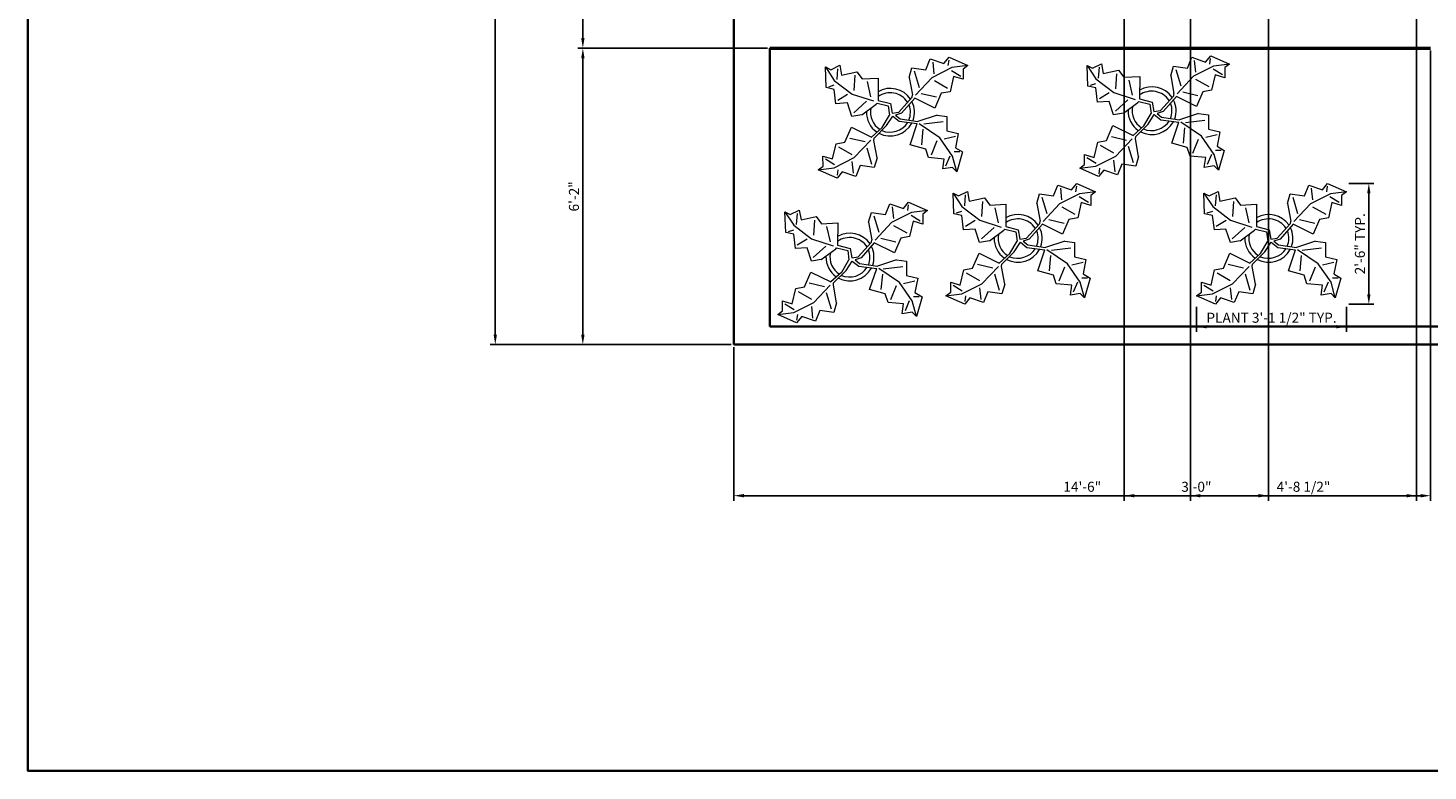
# Model space of a CAD drawing. Units: inches. Extents: x 65 to 818, y -87 to 880.
# Tile 1 of 6: x 65 to 414, y -87 to 98. Entities that reach past the tile are written whole.
import ezdxf

# ---------------------------------------------------------------- set-up
doc = ezdxf.new("R2010")
doc.units = ezdxf.units.IN
for name, color, linetype, lineweight in [('A-ANNO-DIMS', 2, 'Continuous', 18), ('A-ANNO-TTLB', 7, 'Continuous', 35), ('A-WALL', 7, 'Continuous', 50), ('C-PROP', 7, 'Continuous', 35), ('L-PLNT', 94, 'Continuous', 13)]:
    doc.layers.add(name, color=color, linetype=linetype, lineweight=lineweight)
doc.styles.get("Standard").update_dxf_attribs({"font": 'arial.ttf'})
doc.dimstyles.new('ISO-25', dxfattribs={"dimtxt": 2.5, "dimasz": 2.5, "dimexe": 1.25, "dimexo": 0.625, "dimtad": 1, "dimtxsty": 'Standard', "dimcen": 2.5, "dimadec": 0, "dimazin": 0, "dimtfac": 1, "dimtmove": 0, "dimatfit": 3, "dimfxl": 1, "dimarcsym": 0})

# ---------------------------------------------------------------- blocks, each defined once
blk = doc.blocks.new('Plant - Rubber or Philodendron')
for p, q in [((-16.2005, 11.4774), (-13.9899, 8.1064)), ((-16.2005, 11.4774), (-14.8639, 10.7964)), ((-16.0159, 6.3329), (-16.2005, 11.4774)), ((-14.8639, 10.7964), (-12.6195, 11.8975)), ((-13.3174, 8.325), (-13.0735, 11.0065)), ((-12.6195, 11.8975), (-12.1909, 9.4345)), ((4.6914, 8.8812), (5.3859, 11.2828)), ((5.3859, 11.2828), (8.8871, 10.7908)), ((8.8871, 10.7908), (9.9809, 13.4933)), ((9.9809, 13.4933), (13.3837, 12.301)), ((15.3859, 11.3055), (10.3916, 8.7942)), ((10.5828, 12.6946), (10.8893, 9.7953)), ((13.3837, 12.301), (14.68, 13.9039)), ((14.5816, 13.2037), (14.3848, 11.8033)), ((14.68, 13.9039), (19.3848, 11.8146)), ((15.2875, 10.6053), (17.5907, 9.2105)), ((19.3848, 11.8146), (15.3859, 11.3055)), ((19.3848, 11.8146), (18.1868, 10.9119)), ((18.1868, 10.9119), (18.1925, 8.4119)), ((-13.9899, 8.1064), (-9.5434, 4.7185)), ((-12.1909, 9.4345), (-8.3829, 10.3)), ((-8.8369, 9.409), (-9.0894, 5.6095)), ((-8.3829, 10.3), (-7.0549, 8.501)), ((-7.0549, 8.501), (-3.0284, 8.6941)), ((-4.8529, 4.012), (-5.7184, 7.82)), ((-3.0284, 8.6941), (-3.0709, 3.1041)), ((4.6914, 8.8812), (5.5014, 4.4831)), ((5.9878, 10.4842), (7.1971, 6.3869)), ((10.3916, 8.7942), (6.2847, 4.4028)), ((14.2977, 6.1031), (10.9934, 7.9956)), ((15.7909, 9.1065), (14.8995, 5.3044)), ((18.1925, 8.4119), (15.7909, 9.1065)), ((-14.0069, 5.8704), (-16.0159, 6.3329)), ((-15.3434, 6.5514), (-13.9984, 6.9884)), ((-13.5868, 2.2894), (-14.0069, 5.8704)), ((-13.1329, 3.1804), (-10.6614, 4.727)), ((-9.5434, 4.7185), (-4.1917, 2.9888)), ((2.1141, 0.2298), (5.4346, 3.9146)), ((6.1032, 3.6844), (2.8262, -0.031)), ((5.4346, 3.9146), (5.5014, 4.4831)), ((11.1089, 1.1958), (6.1032, 3.6844)), ((7.7005, 4.8881), (11.5025, 3.9967)), ((12.7005, 4.8994), (11.1089, 1.1958)), ((14.8995, 5.3044), (12.7005, 4.8994)), ((-10.6784, 2.491), (-13.5868, 2.2894)), ((-9.5858, -0.8715), (-10.6784, 2.491)), ((-9.1318, 0.0195), (-5.9793, 2.9025)), ((-7.1228, -0.443), (-3.5248, 2.2131)), ((-3.5248, 2.2131), (-3.3011, 2.4355)), ((-3.3011, 2.4355), (-0.5306, 1.7947)), ((-3.0709, 3.1041), (0.0797, 2.3163)), ((-0.5306, 1.7947), (-0.2255, -0.5527)), ((-0.5306, 1.7947), (-0.5306, 1.7947)), ((0.0797, 2.3163), (0.4866, -0.031)), ((0.4866, -0.031), (2.1141, 0.2298)), ((-7.1228, -0.443), (-9.5858, -0.8715)), ((-4.0579, -6.2781), (-0.9375, -3.1608)), ((-2.019, -3.6148), (-0.2255, -0.5527)), ((-0.9375, -3.1608), (0.5883, -0.8135)), ((0.5883, -0.8135), (2.2447, -2.0916)), ((2.8262, -0.031), (1.3003, -0.5527)), ((1.3003, -0.5527), (2.4193, -1.4655)), ((2.2447, -2.0916), (6.7108, -2.6626)), ((2.4193, -1.4655), (6.895, -2.1175)), ((4.943, -7.9659), (6.7108, -2.6626)), ((11.6605, -0.5413), (6.895, -2.1175)), ((12.3677, -6.1981), (7.219, -2.6772)), ((8.3544, -2.7453), (13.1973, -2.1704)), ((11.6605, -0.5413), (14.1354, -0.8948)), ((14.1354, -0.8948), (14.1354, -4.4304)), ((-11.3237, -7.2629), (-9.7321, -3.5593)), ((-6.3237, -7.2516), (-10.1257, -6.3602)), ((-9.7321, -3.5593), (-4.7264, -6.0479)), ((-9.0148, -11.1577), (-4.9047, -6.8122)), ((-2.019, -3.6148), (-4.7264, -6.0479)), ((-4.1246, -6.8466), (-4.0579, -6.2781)), ((-3.3146, -11.2447), (-4.1246, -6.8466)), ((8.125, -4.0768), (7.7715, -7.9659)), ((10.2463, -10.4408), (11.6605, -6.9053)), ((15.5496, -10.7943), (12.3677, -6.1981)), ((16.2567, -5.8446), (13.4283, -6.5517)), ((14.1354, -4.4304), (16.9638, -5.1375)), ((16.9638, -5.1375), (16.2567, -8.673)), ((-14.4141, -11.4699), (-13.5228, -7.6679)), ((-13.5228, -7.6679), (-11.3237, -7.2629)), ((-12.921, -8.4665), (-9.6166, -10.359)), ((-4.611, -12.8477), (-5.8203, -8.7504)), ((8.8321, -9.0266), (4.943, -7.9659)), ((9.5392, -11.1479), (8.8321, -9.0266)), ((17.3174, -9.7337), (15.9032, -9.7337)), ((16.2567, -8.673), (18.0245, -9.7337)), ((18.0245, -9.7337), (16.6103, -14.6834)), ((-18.008, -14.1781), (-16.8101, -13.2754)), ((-18.008, -14.1781), (-14.0091, -13.669)), ((-16.8157, -10.7754), (-14.4141, -11.4699)), ((-16.8101, -13.2754), (-16.8157, -10.7754)), ((-13.9107, -12.9688), (-16.2139, -11.574)), ((-14.0091, -13.669), (-9.0148, -11.1577)), ((-9.206, -15.0581), (-9.5126, -12.1588)), ((-7.5103, -13.1543), (-8.6042, -15.8568)), ((-4.0092, -13.6463), (-7.5103, -13.1543)), ((-3.3146, -11.2447), (-4.0092, -13.6463)), ((13.4283, -11.5015), (9.5392, -11.1479)), ((13.0748, -13.9763), (13.4283, -11.5015)), ((15.5496, -13.6228), (13.0748, -13.9763)), ((14.8425, -10.7943), (13.7819, -13.2692)), ((16.6103, -14.6834), (15.5496, -10.7943)), ((16.6103, -14.6834), (15.5496, -13.6228)), ((-13.3032, -16.2674), (-18.008, -14.1781)), ((-12.0069, -14.6645), (-13.3032, -16.2674)), ((-13.2048, -15.5672), (-13.008, -14.1668)), ((-8.6042, -15.8568), (-12.0069, -14.6645))]:
    blk.add_line(p, q)
for centre, radius, start, end in [((0, 0), 6.1275, 34.37569, 120.1028), ((-0.0601, -0.2075), 5.2461, 33.82192, 124.9414), ((0.0308, 0.1664), 6, 178.6147, 235.1169), ((0.0308, 0.1664), 5, 168.1647, 238.6725), ((-0.2664, 0.1682), 5.2775, 338.4094, 20.03007), ((-0.098, 0.1364), 6.1288, 341.2017, 26.09184), ((-0.0234, 0.3825), 6.1492, 242.5812, 331.2714), ((-0.1102, 0.4886), 5.2883, 247.3711, 327.472)]:
    blk.add_arc(centre, radius, start, end)
blk = doc.blocks.new('*D14')
at = {"layer": 'A-ANNO-DIMS', "color": 0, "lineweight": -2, "transparency": 16777216}
for p, q in [((240.17, 739.04), (179.98, 739.04)), ((181.23, 21.54), (181.23, 736.54)), ((240.17, 19.04), (179.98, 19.04))]:
    blk.add_line(p, q, dxfattribs=at)
at = {"layer": 'A-ANNO-DIMS', "color": 0, "transparency": 16777216}
for points in [[(180.81, 736.54), (181.65, 736.54), (181.23, 739.04)], [(180.81, 21.54), (181.65, 21.54), (181.23, 19.04)]]:
    blk.add_solid(points, dxfattribs=at)
at = {"layer": 'Defpoints', "color": 0, "transparency": 16777216}
for p in [(181.23, 739.04), (240.8, 739.04), (240.8, 19.04)]:
    blk.add_point(p, dxfattribs=at)
at = {"layer": 'A-ANNO-DIMS', "color": 0, "transparency": 16777216, "insert": (180.09, 379.04), "char_height": 1, "attachment_point": 5, "rotation": 90}
blk.add_mtext("60'", dxfattribs=at)
blk = doc.blocks.new('*D20')
at = {"layer": 'A-ANNO-DIMS', "color": 0, "lineweight": -2, "transparency": 16777216}
for p, q in [((356.36, 28.5), (356.36, 22.27)), ((393.75, 28.5), (393.75, 22.27)), ((358.86, 23.52), (391.25, 23.52))]:
    blk.add_line(p, q, dxfattribs=at)
at = {"layer": 'A-ANNO-DIMS', "color": 0, "transparency": 16777216}
for points in [[(358.86, 23.93), (358.86, 23.1), (356.36, 23.52)], [(391.25, 23.93), (391.25, 23.1), (393.75, 23.52)]]:
    blk.add_solid(points, dxfattribs=at)
at = {"layer": 'Defpoints', "color": 0, "transparency": 16777216}
for p in [(356.36, 29.12), (393.75, 29.12), (393.75, 23.52)]:
    blk.add_point(p, dxfattribs=at)
at = {"layer": 'A-ANNO-DIMS', "color": 0, "transparency": 16777216, "insert": (375.06, 25.43), "char_height": 2.5, "attachment_point": 5}
blk.add_mtext('PLANT 3\'-1 1/2" TYP.', dxfattribs=at)
blk = doc.blocks.new('*D21')
at = {"layer": 'A-ANNO-DIMS', "color": 0, "lineweight": -2, "transparency": 16777216}
for p, q in [((394.38, 59.3), (400.61, 59.3)), ((399.36, 31.62), (399.36, 56.8)), ((394.38, 29.12), (400.61, 29.12))]:
    blk.add_line(p, q, dxfattribs=at)
at = {"layer": 'A-ANNO-DIMS', "color": 0, "transparency": 16777216}
for points in [[(398.95, 56.8), (399.78, 56.8), (399.36, 59.3)], [(398.95, 31.62), (399.78, 31.62), (399.36, 29.12)]]:
    blk.add_solid(points, dxfattribs=at)
at = {"layer": 'Defpoints', "color": 0, "transparency": 16777216}
for p in [(393.75, 59.3), (399.36, 59.3), (393.75, 29.12)]:
    blk.add_point(p, dxfattribs=at)
at = {"layer": 'A-ANNO-DIMS', "color": 0, "transparency": 16777216, "insert": (397.46, 44.21), "char_height": 2.5, "attachment_point": 5, "rotation": 90}
blk.add_mtext('2\'-6" TYP.', dxfattribs=at)
blk = doc.blocks.new('*D52')
at = {"layer": 'A-ANNO-DIMS', "color": 0, "lineweight": -2, "transparency": 16777216}
for p, q in [((240.17, 703.04), (201.85, 703.04)), ((203.1, 700.54), (203.1, 95.54)), ((249.17, 93.04), (201.85, 93.04))]:
    blk.add_line(p, q, dxfattribs=at)
at = {"layer": 'A-ANNO-DIMS', "color": 0, "transparency": 16777216}
for points in [[(202.68, 700.54), (203.52, 700.54), (203.1, 703.04)], [(202.68, 95.54), (203.52, 95.54), (203.1, 93.04)]]:
    blk.add_solid(points, dxfattribs=at)
at = {"layer": 'Defpoints', "color": 0, "transparency": 16777216}
for p in [(240.8, 703.04), (203.1, 93.04), (249.8, 93.04)]:
    blk.add_point(p, dxfattribs=at)
at = {"layer": 'A-ANNO-DIMS', "color": 0, "transparency": 16777216, "insert": (201.2, 398.04), "char_height": 2.5, "attachment_point": 5, "rotation": 90}
blk.add_mtext('50\'-10"', dxfattribs=at)
blk = doc.blocks.new('*D53')
at = {"layer": 'A-ANNO-DIMS', "color": 0, "lineweight": -2, "transparency": 16777216}
for p, q in [((249.17, 93.04), (201.85, 93.04)), ((203.1, 90.54), (203.1, 21.54)), ((240.17, 19.04), (201.85, 19.04))]:
    blk.add_line(p, q, dxfattribs=at)
at = {"layer": 'A-ANNO-DIMS', "color": 0, "transparency": 16777216}
for points in [[(202.68, 90.54), (203.52, 90.54), (203.1, 93.04)], [(202.68, 21.54), (203.52, 21.54), (203.1, 19.04)]]:
    blk.add_solid(points, dxfattribs=at)
at = {"layer": 'Defpoints', "color": 0, "transparency": 16777216}
for p in [(249.8, 93.04), (203.1, 19.04), (240.8, 19.04)]:
    blk.add_point(p, dxfattribs=at)
at = {"layer": 'A-ANNO-DIMS', "color": 0, "transparency": 16777216, "insert": (201.2, 56.04), "char_height": 2.5, "attachment_point": 5, "rotation": 90}
blk.add_mtext('6\'-2"', dxfattribs=at)
blk = doc.blocks.new('*D71')
at = {"layer": 'A-ANNO-DIMS', "color": 0, "lineweight": -2, "transparency": 16777216}
for p, q in [((414.8, 92.42), (414.8, -19.91)), ((240.8, 18.42), (240.8, -19.91)), ((243.3, -18.66), (412.3, -18.66))]:
    blk.add_line(p, q, dxfattribs=at)
at = {"layer": 'A-ANNO-DIMS', "color": 0, "transparency": 16777216}
for points in [[(243.3, -18.25), (243.3, -19.08), (240.8, -18.66)], [(412.3, -18.25), (412.3, -19.08), (414.8, -18.66)]]:
    blk.add_solid(points, dxfattribs=at)
at = {"layer": 'Defpoints', "color": 0, "transparency": 16777216}
for p in [(414.8, 93.04), (240.8, 19.04), (414.8, -18.66)]:
    blk.add_point(p, dxfattribs=at)
at = {"layer": 'A-ANNO-DIMS', "color": 0, "transparency": 16777216, "insert": (327.8, -16.76), "char_height": 2.5, "attachment_point": 5}
blk.add_mtext('14\'-6"', dxfattribs=at)
blk = doc.blocks.new('*D72')
at = {"layer": 'A-ANNO-DIMS', "color": 0, "lineweight": -2, "transparency": 16777216}
for p, q in [((354.8, 498.42), (354.8, -19.91)), ((411.3, 498.42), (411.3, -19.91)), ((357.3, -18.66), (408.8, -18.66))]:
    blk.add_line(p, q, dxfattribs=at)
at = {"layer": 'A-ANNO-DIMS', "color": 0, "transparency": 16777216}
for points in [[(357.3, -18.25), (357.3, -19.08), (354.8, -18.66)], [(408.8, -18.25), (408.8, -19.08), (411.3, -18.66)]]:
    blk.add_solid(points, dxfattribs=at)
at = {"layer": 'Defpoints', "color": 0, "transparency": 16777216}
for p in [(354.8, 499.04), (411.3, 499.04), (411.3, -18.66)]:
    blk.add_point(p, dxfattribs=at)
at = {"layer": 'A-ANNO-DIMS', "color": 0, "transparency": 16777216, "insert": (383.05, -16.75), "char_height": 2.5, "attachment_point": 5}
blk.add_mtext('4\'-8 1/2"', dxfattribs=at)
blk = doc.blocks.new('*D73')
at = {"layer": 'A-ANNO-DIMS', "color": 0, "lineweight": -2, "transparency": 16777216}
for p, q in [((338.3, 360.42), (338.3, -19.91)), ((374.3, 360.42), (374.3, -19.91)), ((340.8, -18.66), (371.8, -18.66))]:
    blk.add_line(p, q, dxfattribs=at)
at = {"layer": 'A-ANNO-DIMS', "color": 0, "transparency": 16777216}
for points in [[(340.8, -18.25), (340.8, -19.08), (338.3, -18.66)], [(371.8, -18.25), (371.8, -19.08), (374.3, -18.66)]]:
    blk.add_solid(points, dxfattribs=at)
at = {"layer": 'Defpoints', "color": 0, "transparency": 16777216}
for p in [(338.3, 361.04), (374.3, 361.04), (374.3, -18.66)]:
    blk.add_point(p, dxfattribs=at)
at = {"layer": 'A-ANNO-DIMS', "color": 0, "transparency": 16777216, "insert": (356.3, -16.76), "char_height": 2.5, "attachment_point": 5}
blk.add_mtext('3\'-0"', dxfattribs=at)

msp = doc.modelspace()

# ---------------------------------------------------------------- linework, layer by layer
at = {"layer": 'A-ANNO-TTLB'}
msp.add_lwpolyline([(64.55, 880.46), (817.59, 880.46), (817.59, -87.37), (64.55, -87.37)], close=True, dxfattribs=at)
at = {"layer": 'A-WALL'}
msp.add_line((249.8, 93.04), (414.8, 93.04), dxfattribs=at)
at = {"layer": 'C-PROP'}
for p, q in [((240.8, 19.04), (240.8, 739.04)), ((249.8, 23.54), (249.8, 93.04)), ((625.16, 23.54), (249.8, 23.54)), ((720.8, 19.04), (240.8, 19.04))]:
    msp.add_line(p, q, dxfattribs=at)

# ---------------------------------------------------------------- block references
at = {"layer": 'L-PLNT'}
for p in [(345.2, 77.26), (279.88, 76.87), (311.76, 45.39), (374.37, 45.39), (269.77, 40.73)]:
    msp.add_blockref('Plant - Rubber or Philodendron', p, dxfattribs=at)

# ---------------------------------------------------------------- dimensions: what is measured, and where the dimension line sits
at = {"layer": 'A-ANNO-DIMS'}
for base, p1, p2, override, picture, middle in [((181.23, 739.04), (240.8, 19.04), (240.8, 739.04), {"dimtxt": 1, "dimdec": 0, "dimlunit": 3, "dimclrd": 0, "dimclre": 0, "dimclrt": 0, "dimtdec": 0}, '*D14', (180.09, 379.04)), ((203.1, 93.04), (240.8, 703.04), (249.8, 93.04), {"dimdec": 1, "dimlfac": 1, "dimrnd": 0, "dimzin": 1, "dimdsep": 46, "dimlunit": 4, "dimfrac": 2}, '*D52', (201.2, 398.04)), ((203.1, 19.04), (249.8, 93.04), (240.8, 19.04), {"dimdec": 1, "dimlfac": 1, "dimrnd": 0, "dimzin": 1, "dimdsep": 46, "dimlunit": 4, "dimfrac": 2}, '*D53', (201.2, 56.04))]:
    dim = msp.add_linear_dim(base=base, p1=p1, p2=p2, angle=90, dimstyle='ISO-25', override=override, dxfattribs=at)
    dim.commit()
    dim.dimension.update_dxf_attribs({"geometry": picture, "text_midpoint": middle})
for base, p1, p2, picture, middle in [((411.3, -18.66), (354.8, 499.04), (411.3, 499.04), '*D72', (383.05, -16.75)), ((374.3, -18.66), (338.3, 361.04), (374.3, 361.04), '*D73', (356.3, -16.76)), ((414.8, -18.66), (240.8, 19.04), (414.8, 93.04), '*D71', (327.8, -16.76))]:
    dim = msp.add_linear_dim(base=base, p1=p1, p2=p2, dimstyle='ISO-25', override={"dimdec": 1, "dimlfac": 1, "dimrnd": 0, "dimzin": 1, "dimdsep": 46, "dimlunit": 4, "dimfrac": 2}, dxfattribs=at)
    dim.commit()
    dim.dimension.update_dxf_attribs({"geometry": picture, "text_midpoint": middle})
dim = msp.add_linear_dim(base=(399.36, 59.3), p1=(393.75, 29.12), p2=(393.75, 59.3), angle=90, text='<> TYP.', dimstyle='ISO-25', override={"dimdec": 1, "dimlfac": 1, "dimrnd": 0, "dimzin": 1, "dimdsep": 46, "dimlunit": 4, "dimfrac": 2}, dxfattribs=at)
dim.commit()
dim.dimension.update_dxf_attribs({"geometry": '*D21', "text_midpoint": (397.46, 44.21)})
dim = msp.add_linear_dim(base=(393.75, 23.52), p1=(356.36, 29.12), p2=(393.75, 29.12), text='PLANT <> TYP.', dimstyle='ISO-25', override={"dimdec": 1, "dimlfac": 1, "dimrnd": 0, "dimzin": 1, "dimdsep": 46, "dimlunit": 4, "dimfrac": 2}, dxfattribs=at)
dim.commit()
dim.dimension.update_dxf_attribs({"geometry": '*D20', "text_midpoint": (375.06, 25.43)})

doc.saveas('drawing.dxf')
